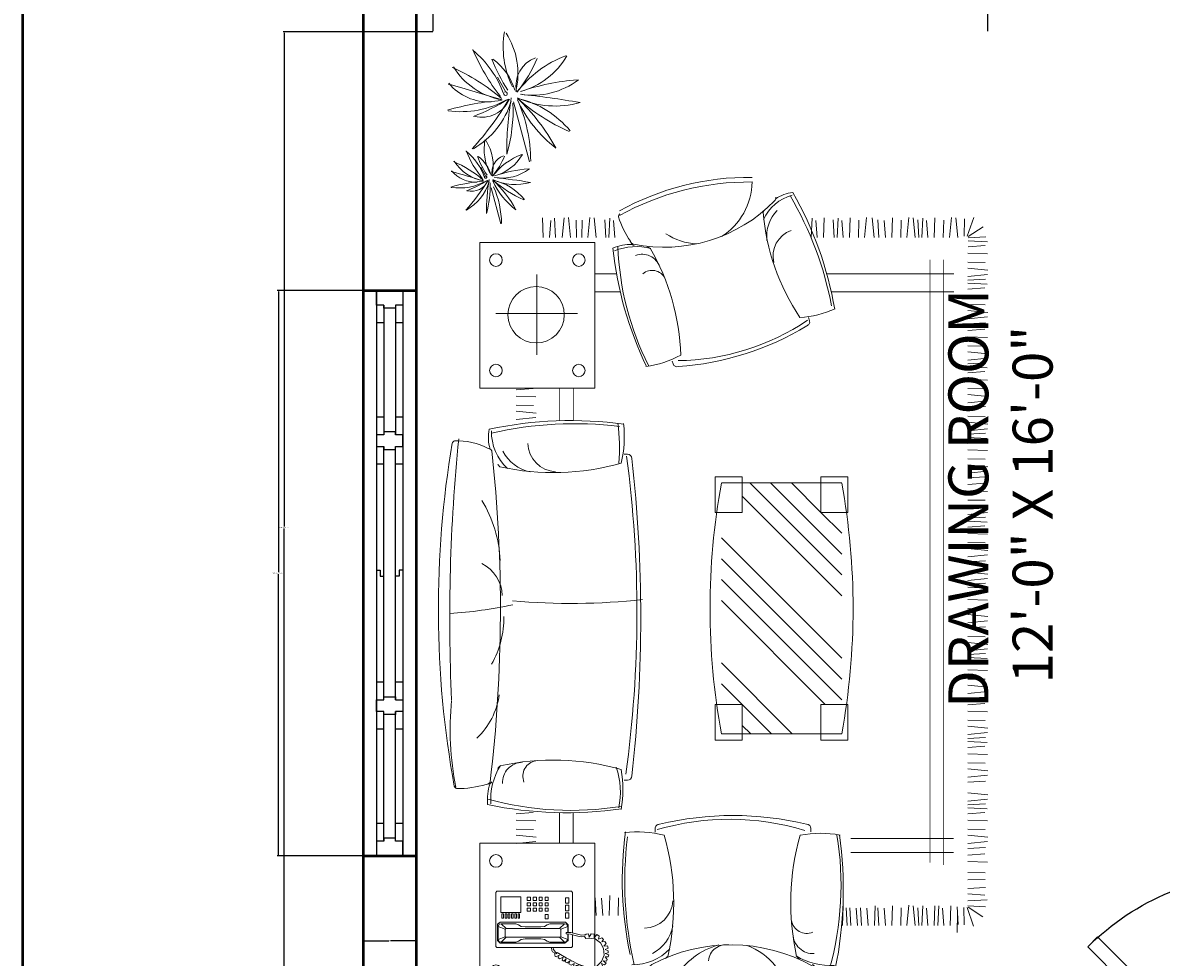
# Model space of a CAD drawing. Units: inches. Extents: x 64 to 1167, y 117 to 939.
# Tile 2 of 56: x 64 to 258, y 272 to 431. Entities that reach past the tile are written whole.
import ezdxf

# ---------------------------------------------------------------- set-up
doc = ezdxf.new("R2010")
doc.units = ezdxf.units.IN
doc.header["$MEASUREMENT"] = 0
for name, color, linetype, lineweight in [('A-ANNO-DIMS', 2, 'Continuous', 18), ('A-ANNO-TEXT', 7, 'Continuous', 25), ('A-ANNO-TTLB', 7, 'Continuous', 50), ('A-DOOR', 4, 'Continuous', 25), ('A-FURN', 8, 'Continuous', 18), ('A-GLAZ', 4, 'Continuous', 25), ('A-WALL', 7, 'Continuous', 50)]:
    doc.layers.add(name, color=color, linetype=linetype, lineweight=lineweight)
doc.styles.get("Standard").update_dxf_attribs({"font": 'arial.ttf'})
doc.dimstyles.get("Standard").update_dxf_attribs({"dimtxt": 0.18, "dimasz": 0.18, "dimexe": 0.18, "dimexo": 0.0625, "dimgap": 0.09, "dimtad": 0, "dimtih": 1, "dimtoh": 1, "dimdec": 4, "dimzin": 0, "dimdsep": 46, "dimtxsty": 'Standard', "dimcen": 0.09, "dimadec": 0, "dimazin": 0, "dimtfac": 1, "dimtdec": 4, "dimtofl": 0, "dimtmove": 0, "dimatfit": 3, "dimfxl": 1, "dimtolj": 1, "dimtzin": 0, "dimarcsym": 0})

# ---------------------------------------------------------------- blocks, each defined once
blk = doc.blocks.new('A$C68901CC0')
for p, q in [((10.95, 26.62), (12.35, 28.01)), ((12.35, 28.01), (37.4, 2.95)), ((36.01, 1.56), (10.95, 26.62)), ((0, 2.95), (0, 0)), ((1.97, 2.95), (0, 2.95)), ((1.97, 0), (1.97, 2.95)), ((37.4, 2.95), (36.01, 1.56)), ((37.4, 2.95), (37.4, 0)), ((39.37, 2.95), (37.4, 2.95)), ((39.37, 0), (39.37, 2.95)), ((0, 0), (1.97, 0)), ((37.4, 0), (39.37, 0))]:
    blk.add_line(p, q)
blk.add_arc((37.4, 2.95), 35.43, 135, 180)
blk = doc.blocks.new("W-8'")
for p, q in [((0, 9), (96, 9)), ((0, 9), (0, 0)), ((96, 9), (96, 0)), ((0, 6.75), (96, 6.75)), ((2.5, 5.5), (24.5, 5.5)), ((69.5, 5.5), (26.5, 5.5)), ((93.5, 5.5), (71.5, 5.5)), ((0, 2.25), (96, 2.25)), ((2.5, 3.5), (24.5, 3.5)), ((69.5, 3.5), (26.5, 3.5)), ((93.5, 3.5), (71.5, 3.5)), ((0, 0), (96, 0))]:
    blk.add_line(p, q)
for points in [[(0, 2.25), (0, 6.75), (2.5, 6.75), (2.5, 5.5), (3, 5.5), (3, 3.5), (2.5, 3.5), (2.5, 2.25), (0, 2.25)], [(5.5, 6.75), (5.5, 5.5)], [(21.5, 6.75), (21.5, 5.5)], [(29.5, 6.75), (29.5, 5.5)], [(47.5, 6.75), (47.5, 6.125), (48.5, 6.125), (48.5, 5.5)], [(66.5, 6.75), (66.5, 5.5)], [(74.5, 6.75), (74.5, 5.5)], [(90.5, 6.75), (90.5, 5.5)], [(96, 2.25), (96, 6.75), (93.5, 6.75), (93.5, 5.5), (93, 5.5), (93, 3.5), (93.5, 3.5), (93.5, 2.25), (96, 2.25)], [(5.5, 3.5), (5.5, 2.25)], [(21.5, 3.5), (21.5, 2.25)], [(29.5, 3.5), (29.5, 2.25)], [(47.5, 2.25), (47.5, 2.875), (48.5, 2.875), (48.5, 3.5)], [(66.5, 3.5), (66.5, 2.25)], [(74.5, 3.5), (74.5, 2.25)], [(90.5, 3.5), (90.5, 2.25)]]:
    blk.add_lwpolyline(points)
for points in [[(26.5, 6.75), (24.5, 6.75), (24.5, 5.5), (24, 5.5), (24, 3.5), (24.5, 3.5), (24.5, 2.25), (26.5, 2.25), (26.5, 3.5), (27, 3.5), (27, 5.5), (26.5, 5.5)], [(69.5, 6.75), (71.5, 6.75), (71.5, 5.5), (72, 5.5), (72, 3.5), (71.5, 3.5), (71.5, 2.25), (69.5, 2.25), (69.5, 3.5), (69, 3.5), (69, 5.5), (69.5, 5.5)]]:
    blk.add_lwpolyline(points, close=True)
blk = doc.blocks.new('A$C28C76B35')
for p, q in [((66.74, 162.49, -24.36), (86.28, 162.49, -24.36)), ((66.74, 137.72, -24.36), (66.74, 162.49, -24.36)), ((86.28, 162.49, -24.36), (86.28, 137.72, -24.36)), ((65.39, 158.69, -55.71), (65.61, 158.93, -55.71)), ((65.61, 158.17, -55.71), (65.39, 158.69, -55.71)), ((65.61, 158.93, -55.71), (66.11, 158.67, -55.71)), ((66.43, 158.63, -55.71), (65.63, 157.82, -55.71)), ((65.94, 159.21, -55.71), (66.32, 159.36, -55.71)), ((66.11, 158.67, -55.71), (65.94, 159.21, -55.71)), ((66.32, 159.36, -55.71), (66.82, 158.91, -55.71)), ((67.82, 158.89, -55.71), (66.43, 158.63, -55.71)), ((66.79, 159.49, 50.88), (67.17, 159.56, 50.88)), ((66.82, 158.91, -55.71), (66.8, 159.49, -55.71)), ((67.17, 159.56, -55.71), (67.45, 159.08, -55.71)), ((67.45, 159.08, -55.71), (67.62, 159.65, -55.71)), ((67.61, 159.66, 50.88), (68.08, 159.57, 50.88)), ((69.56, 158.28, -55.71), (67.82, 158.89, -55.71)), ((68.08, 159.56, -55.71), (68.08, 159.06, -55.71)), ((68.08, 159.06, -55.71), (68.45, 159.45, -55.71)), ((68.44, 159.45, 50.88), (68.87, 159.32, 50.88)), ((68.88, 159.32, -55.71), (68.86, 158.73, -55.71)), ((68.86, 158.73, -55.71), (69.06, 159.26, -55.71)), ((69.06, 159.26, -55.71), (69.62, 159.1, -55.71)), ((69.62, 159.1, -55.71), (69.56, 158.54, -55.71)), ((69.56, 158.54, -55.71), (70.1, 158.87, -55.71)), ((70.1, 158.87, -55.71), (70.4, 158.67, -55.71)), ((70.4, 158.67, -55.71), (70.25, 158.15, -55.71)), ((64.4, 156.67, -55.71), (64.5, 157.02, -55.71)), ((65, 156.46, -55.71), (64.4, 156.67, -55.71)), ((64.5, 157.02, -55.71), (65, 157.04, -55.71)), ((64.63, 157.46, -55.71), (64.77, 157.76, -55.71)), ((65, 157.04, -55.71), (64.63, 157.46, -55.71)), ((64.77, 157.76, -55.71), (65.33, 157.7, -55.71)), ((64.85, 158.09, -55.71), (65.11, 158.39, -55.71)), ((65.33, 157.7, -55.71), (64.85, 158.09, -55.71)), ((65.11, 158.39, -55.71), (65.61, 158.17, -55.71)), ((65.63, 157.82, -55.71), (65.16, 156.74, -55.71)), ((65.16, 156.74, -55.71), (65.26, 155.63, -55.71)), ((70.64, 157.69, -55.71), (69.56, 158.28, -55.71)), ((70.25, 158.15, -55.71), (70.75, 158.43, -55.71)), ((70.79, 157.74, -55.71), (70.64, 157.69, -55.71)), ((70.75, 158.43, -55.71), (71.14, 158.22, -55.71)), ((70.83, 157.61, -55.71), (70.79, 157.74, -55.71)), ((71.59, 157.22, -55.71), (70.83, 157.61, -55.71)), ((71.14, 158.22, -55.71), (70.98, 157.72, -55.71)), ((70.98, 157.72, -55.71), (71.4, 158.06, -55.71)), ((71.4, 158.06, -55.71), (71.81, 157.87, -55.71)), ((71.81, 157.87, -55.71), (71.59, 157.37, -55.71)), ((71.59, 157.37, -55.71), (72.01, 157.76, -55.71)), ((72.59, 156.63, -55.71), (71.59, 157.22, -55.71)), ((72.01, 157.76, -55.71), (72.31, 157.61, -55.71)), ((72.31, 157.61, -55.71), (72.14, 157.07, -55.71)), ((72.14, 157.07, -55.71), (72.68, 157.37, -55.71)), ((73.15, 156.29, -55.71), (72.59, 156.63, -55.71)), ((72.68, 157.37, -55.71), (72.96, 157.22, -55.71)), ((72.96, 157.22, -55.71), (72.81, 156.74, -55.71)), ((72.81, 156.74, -55.71), (73.3, 157.04, -55.71)), ((73.3, 157.04, -55.71), (73.5, 156.96, -55.71)), ((73.5, 156.96, -55.71), (73.56, 156.76, -55.71)), ((73.56, 156.76, -55.71), (73.57, 156.42, -55.71)), ((64.46, 156.33, -55.71), (65, 156.46, -55.71)), ((64.5, 156.02, -55.71), (64.46, 156.33, -55.71)), ((65, 155.79, -55.71), (64.5, 156.02, -55.71)), ((64.5, 155.55, -55.71), (65, 155.79, -55.71)), ((64.61, 155.16, -55.71), (64.5, 155.55, -55.71)), ((65.22, 155.22, -55.71), (64.61, 155.16, -55.71)), ((64.85, 154.77, -55.71), (65.22, 155.22, -55.71)), ((65.07, 154.42, -55.71), (64.85, 154.77, -55.71)), ((65.26, 155.63, -55.71), (65.78, 154.64, -55.71)), ((65.78, 154.64, -55.71), (66.67, 153.94, -55.71)), ((70.72, 155.44, -55.71), (70.54, 155.25, -55.71)), ((70.54, 155.25, -55.71), (70.54, 153.28, -55.71)), ((83.37, 155.44, -55.71), (70.72, 155.44, -55.71)), ((71.82, 154.7, -55.71), (71.27, 154.24, -55.71)), ((82.82, 154.7, -55.71), (71.82, 154.7, -55.71)), ((73.33, 156.52, -55.71), (73.15, 156.29, -55.71)), ((73.33, 156.33, -55.71), (73.33, 156.52, -55.71)), ((73.44, 156.22, -55.71), (73.33, 156.33, -55.71)), ((73.61, 155.98, -55.71), (73.44, 156.22, -55.71)), ((73.57, 156.42, -55.71), (73.93, 156.16, -55.71)), ((73.76, 155.78, -55.71), (73.61, 155.98, -55.71)), ((73.84, 155.44, -55.71), (73.76, 155.78, -55.71)), ((73.93, 156.16, -55.71), (74.06, 155.94, -55.71)), ((74.06, 155.94, -55.71), (74.11, 155.44, -55.71)), ((83.28, 154.24, -55.71), (82.82, 154.7, -55.71)), ((83.55, 155.25, -55.71), (83.37, 155.44, -55.71)), ((83.55, 146.08, -55.71), (83.55, 155.25, -55.71)), ((5.16, 149.65, -28.15), (5.22, 152.89, -28.15)), ((65.57, 154.5, -55.71), (65.07, 154.42, -55.71)), ((65.26, 154.07, -55.71), (65.57, 154.5, -55.71)), ((65.59, 153.79, -55.71), (65.26, 154.07, -55.71)), ((66.11, 154.05, -55.71), (65.59, 153.79, -55.71)), ((66, 153.49, -55.71), (66.11, 154.05, -55.71)), ((66.43, 153.25, -55.71), (66, 153.49, -55.71)), ((66.84, 153.77, -55.71), (66.43, 153.25, -55.71)), ((66.67, 153.94, -55.71), (67.84, 153.85, -55.71)), ((66.89, 153.18, -55.71), (66.84, 153.77, -55.71)), ((67.39, 153.14, -55.71), (66.89, 153.18, -55.71)), ((67.71, 153.66, -55.71), (67.39, 153.14, -55.71)), ((67.8, 153.12, -55.71), (67.71, 153.66, -55.71)), ((68.25, 153.16, -55.71), (67.8, 153.12, -55.71)), ((67.84, 153.85, -55.71), (68.26, 153.92, -55.71)), ((68.45, 153.36, -55.71), (68.25, 153.16, -55.71)), ((68.26, 153.92, -55.71), (68.51, 153.59, -55.71)), ((68.56, 153.31, -55.71), (68.45, 153.36, -55.71)), ((68.51, 153.59, -55.71), (68.99, 153.6, -55.71)), ((69.04, 153.33, -55.71), (68.56, 153.31, -55.71)), ((68.99, 153.6, -55.71), (69.43, 153.55, -55.71)), ((69.92, 153.1, -55.71), (69.04, 153.33, -55.71)), ((69.43, 153.55, -55.71), (70.31, 153.33, -55.71)), ((70.85, 152.88, -55.71), (69.92, 153.1, -55.71)), ((70.31, 153.33, -55.71), (70.9, 153.2, -55.71)), ((70.54, 152.96, -55.71), (70.54, 146.08, -55.71)), ((71.64, 152.87, -55.71), (70.85, 152.88, -55.71)), ((70.9, 153.2, -55.71), (71.64, 153.14, -55.71)), ((71.27, 154.24, -55.71), (71.27, 153.17, -55.71)), ((71.27, 152.87, -55.71), (71.27, 151.58, -55.71)), ((71.36, 154.06, -55.71), (71.54, 154.43, -55.71)), ((71.36, 153.16, -55.71), (71.36, 154.06, -55.71)), ((72.55, 153.6, -55.71), (71.36, 154.06, -55.71)), ((71.36, 151.86, -55.71), (71.36, 152.87, -55.71)), ((71.54, 154.43, -55.71), (71.91, 154.52, -55.71)), ((71.64, 153.14, -55.71), (71.64, 152.87, -55.71)), ((71.91, 154.52, -55.71), (74.39, 154.52, -55.71)), ((71.91, 154.52, -55.71), (72.74, 153.69, -55.71)), ((72.74, 153.69, -55.71), (72.55, 153.6, -55.71)), ((72.55, 153.6, -55.71), (72.55, 152.32, -55.71)), ((77.69, 153.69, -55.71), (72.74, 153.69, -55.71)), ((74.39, 154.52, -55.71), (74.84, 154.34, -55.71)), ((74.84, 154.34, -55.71), (75.3, 154.06, -55.71)), ((75.3, 154.06, -55.71), (75.94, 153.97, -55.71)), ((75.94, 153.97, -55.71), (77.69, 153.97, -55.71)), ((78.6, 153.97, -55.71), (77.69, 153.97, -55.71)), ((77.69, 153.69, -55.71), (81.81, 153.69, -55.71)), ((79.24, 154.06, -55.71), (78.6, 153.97, -55.71)), ((79.7, 154.34, -55.71), (79.24, 154.06, -55.71)), ((80.16, 154.52, -55.71), (79.7, 154.34, -55.71)), ((82.64, 154.52, -55.71), (80.16, 154.52, -55.71)), ((82.64, 154.52, -55.71), (81.81, 153.69, -55.71)), ((81.81, 153.69, -55.71), (82, 153.6, -55.71)), ((82, 153.6, -55.71), (83.19, 154.06, -55.71)), ((82, 153.6, -55.71), (82, 152.32, -55.71)), ((83, 154.43, -55.71), (82.64, 154.52, -55.71)), ((83.19, 154.06, -55.71), (83, 154.43, -55.71)), ((83.19, 151.86, -55.71), (83.19, 154.06, -55.71)), ((83.28, 151.49, -55.71), (83.28, 154.24, -55.71)), ((3.54, 148.64, -28.15), (2.43, 151.81, -28.15)), ((4.08, 148.65, -28.15), (4.03, 151.6, -28.15)), ((5.25, 148.56, -28.15), (5.08, 151.56, -28.15)), ((6.41, 151.68, -28.15), (6.3, 148.34, -28.15)), ((7.49, 151.68, -28.15), (7.72, 148.79, -28.15)), ((8.51, 151.68, -28.15), (8.34, 148.39, -28.15)), ((9.11, 151.68, -28.15), (9, 148.34, -28.15)), ((10.19, 151.68, -28.15), (10.42, 148.79, -28.15)), ((11.21, 151.68, -28.15), (11.04, 148.39, -28.15)), ((11.72, 151.68, -28.15), (11.89, 148.68, -28.15)), ((12.34, 151.68, -28.15), (12.68, 148.34, -28.15)), ((13.76, 151.68, -28.15), (13.42, 148.28, -28.15)), ((14.78, 151.68, -28.15), (14.72, 148.73, -28.15)), ((16.31, 151.68, -28.15), (16.2, 148.34, -28.15)), ((17.39, 151.68, -28.15), (17.62, 148.79, -28.15)), ((18.52, 151.68, -28.15), (18.69, 148.68, -28.15)), ((19.28, 151.68, -28.15), (19.17, 148.34, -28.15)), ((20.36, 151.68, -28.15), (20.59, 148.79, -28.15)), ((21.49, 151.68, -28.15), (21.66, 148.68, -28.15)), ((22.16, 151.68, -28.15), (22.38, 148.79, -28.15)), ((23.29, 151.68, -28.15), (23.46, 148.68, -28.15)), ((23.92, 151.68, -28.15), (24.09, 148.68, -28.15)), ((24.68, 151.68, -28.15), (24.56, 148.34, -28.15)), ((71.27, 151.58, -55.71), (71.73, 151.13, -55.71)), ((72.55, 152.32, -55.71), (71.36, 151.86, -55.71)), ((71.36, 151.86, -55.71), (71.54, 151.49, -55.71)), ((71.54, 151.49, -55.71), (71.91, 151.4, -55.71)), ((71.73, 151.13, -55.71), (82.82, 151.13, -55.71)), ((71.91, 151.4, -55.71), (72.74, 152.23, -55.71)), ((71.91, 151.4, -55.71), (74.39, 151.4, -55.71)), ((72.74, 152.23, -55.71), (72.55, 152.32, -55.71)), ((77.69, 152.23, -55.71), (72.74, 152.23, -55.71)), ((74.39, 151.4, -55.71), (74.84, 151.58, -55.71)), ((74.84, 151.58, -55.71), (75.3, 151.86, -55.71)), ((75.3, 151.86, -55.71), (75.94, 151.95, -55.71)), ((75.94, 151.95, -55.71), (77.69, 151.95, -55.71)), ((77.69, 152.23, -55.71), (81.81, 152.23, -55.71)), ((78.6, 151.95, -55.71), (77.69, 151.95, -55.71)), ((79.24, 151.86, -55.71), (78.6, 151.95, -55.71)), ((79.7, 151.58, -55.71), (79.24, 151.86, -55.71)), ((80.16, 151.4, -55.71), (79.7, 151.58, -55.71)), ((82.64, 151.4, -55.71), (80.16, 151.4, -55.71)), ((81.81, 152.23, -55.71), (82, 152.32, -55.71)), ((82.64, 151.4, -55.71), (81.81, 152.23, -55.71)), ((82, 152.32, -55.71), (83.19, 151.86, -55.71)), ((83, 151.49, -55.71), (82.64, 151.4, -55.71)), ((82.82, 151.13, -55.71), (83.28, 151.49, -55.71)), ((83.19, 151.86, -55.71), (83, 151.49, -55.71)), ((3.38, 148.57, -28.15), (0.87, 150.22, -28.15)), ((62.8, 149.98, -28.15), (62.74, 147.03, -28.15)), ((64.33, 149.98, -28.15), (64.22, 146.64, -28.15)), ((65.41, 149.98, -28.15), (65.64, 147.09, -28.15)), ((66.54, 149.98, -28.15), (66.71, 146.98, -28.15)), ((71.18, 150.48, -55.71), (71.73, 150.48, -55.71)), ((71.18, 149.57, -55.71), (71.18, 150.48, -55.71)), ((71.73, 149.57, -55.71), (71.18, 149.57, -55.71)), ((71.18, 149.2, -55.71), (71.73, 149.2, -55.71)), ((71.18, 148.28, -55.71), (71.18, 149.2, -55.71)), ((71.73, 150.48, -55.71), (71.73, 149.57, -55.71)), ((71.73, 149.2, -55.71), (71.73, 148.28, -55.71)), ((75.21, 150.58, -55.71), (74.66, 150.58, -55.71)), ((74.66, 150.58, -55.71), (74.66, 149.84, -55.71)), ((74.66, 149.84, -55.71), (75.21, 149.84, -55.71)), ((75.21, 149.29, -55.71), (74.66, 149.29, -55.71)), ((74.66, 149.29, -55.71), (74.66, 148.74, -55.71)), ((75.21, 149.84, -55.71), (75.21, 150.58, -55.71)), ((75.21, 148.74, -55.71), (75.21, 149.29, -55.71)), ((76.22, 149.29, -55.71), (75.67, 149.29, -55.71)), ((75.67, 149.29, -55.71), (75.67, 148.74, -55.71)), ((76.22, 148.74, -55.71), (76.22, 149.29, -55.71)), ((77.23, 149.29, -55.71), (76.68, 149.29, -55.71)), ((76.68, 149.29, -55.71), (76.68, 148.74, -55.71)), ((77.23, 148.74, -55.71), (77.23, 149.29, -55.71)), ((78.24, 149.29, -55.71), (77.69, 149.29, -55.71)), ((77.69, 149.29, -55.71), (77.69, 148.74, -55.71)), ((78.24, 148.74, -55.71), (78.24, 149.29, -55.71)), ((82.73, 149.48, -55.71), (79.34, 149.48, -55.71)), ((79.34, 149.48, -55.71), (79.34, 146.82, -55.71)), ((79.52, 150.48, -55.71), (79.79, 150.48, -55.71)), ((79.52, 149.75, -55.71), (79.52, 150.48, -55.71)), ((79.79, 149.75, -55.71), (79.52, 149.75, -55.71)), ((79.79, 150.48, -55.71), (79.79, 149.75, -55.71)), ((80.07, 150.48, -55.71), (80.35, 150.48, -55.71)), ((80.07, 149.75, -55.71), (80.07, 150.48, -55.71)), ((80.35, 149.75, -55.71), (80.07, 149.75, -55.71)), ((80.35, 150.48, -55.71), (80.35, 149.75, -55.71)), ((80.62, 150.48, -55.71), (80.9, 150.48, -55.71)), ((80.62, 149.75, -55.71), (80.62, 150.48, -55.71)), ((80.9, 149.75, -55.71), (80.62, 149.75, -55.71)), ((80.9, 150.48, -55.71), (80.9, 149.75, -55.71)), ((81.17, 150.48, -55.71), (81.45, 150.48, -55.71)), ((81.17, 149.75, -55.71), (81.17, 150.48, -55.71)), ((81.45, 149.75, -55.71), (81.17, 149.75, -55.71)), ((81.45, 150.48, -55.71), (81.45, 149.75, -55.71)), ((81.72, 150.48, -55.71), (82, 150.48, -55.71)), ((81.72, 149.75, -55.71), (81.72, 150.48, -55.71)), ((82, 149.75, -55.71), (81.72, 149.75, -55.71)), ((82, 150.48, -55.71), (82, 149.75, -55.71)), ((82.27, 150.48, -55.71), (82.55, 150.48, -55.71)), ((82.27, 149.75, -55.71), (82.27, 150.48, -55.71)), ((82.55, 149.75, -55.71), (82.27, 149.75, -55.71)), ((82.55, 150.48, -55.71), (82.55, 149.75, -55.71)), ((82.73, 146.82, -55.71), (82.73, 149.48, -55.71)), ((3.4, 147.54, -28.15), (0.11, 147.37, -28.15)), ((3.4, 148.35, -28.15), (0.4, 148.52, -28.15)), ((71.73, 148.28, -55.71), (71.18, 148.28, -55.71)), ((71.18, 147.92, -55.71), (71.73, 147.92, -55.71)), ((71.18, 147, -55.71), (71.18, 147.92, -55.71)), ((71.73, 147, -55.71), (71.18, 147, -55.71)), ((71.73, 147.92, -55.71), (71.73, 147, -55.71)), ((74.66, 148.74, -55.71), (75.21, 148.74, -55.71)), ((74.66, 148.38, -55.71), (74.66, 147.83, -55.71)), ((75.21, 148.38, -55.71), (74.66, 148.38, -55.71)), ((74.66, 147.83, -55.71), (75.21, 147.83, -55.71)), ((75.21, 147.46, -55.71), (74.66, 147.46, -55.71)), ((74.66, 147.46, -55.71), (74.66, 146.91, -55.71)), ((74.66, 146.91, -55.71), (75.21, 146.91, -55.71)), ((75.21, 147.83, -55.71), (75.21, 148.38, -55.71)), ((75.21, 146.91, -55.71), (75.21, 147.46, -55.71)), ((75.67, 148.74, -55.71), (76.22, 148.74, -55.71)), ((75.67, 148.38, -55.71), (75.67, 147.83, -55.71)), ((76.22, 148.38, -55.71), (75.67, 148.38, -55.71)), ((75.67, 147.83, -55.71), (76.22, 147.83, -55.71)), ((76.22, 147.46, -55.71), (75.67, 147.46, -55.71)), ((75.67, 147.46, -55.71), (75.67, 146.91, -55.71)), ((75.67, 146.91, -55.71), (76.22, 146.91, -55.71)), ((76.22, 147.83, -55.71), (76.22, 148.38, -55.71)), ((76.22, 146.91, -55.71), (76.22, 147.46, -55.71)), ((76.68, 148.74, -55.71), (77.23, 148.74, -55.71)), ((77.23, 148.38, -55.71), (76.68, 148.38, -55.71)), ((76.68, 148.38, -55.71), (76.68, 147.83, -55.71)), ((76.68, 147.83, -55.71), (77.23, 147.83, -55.71)), ((77.23, 147.46, -55.71), (76.68, 147.46, -55.71)), ((76.68, 147.46, -55.71), (76.68, 146.91, -55.71)), ((76.68, 146.91, -55.71), (77.23, 146.91, -55.71)), ((77.23, 147.83, -55.71), (77.23, 148.38, -55.71)), ((77.23, 146.91, -55.71), (77.23, 147.46, -55.71)), ((77.69, 148.74, -55.71), (78.24, 148.74, -55.71)), ((77.69, 148.38, -55.71), (77.69, 147.83, -55.71)), ((78.24, 148.38, -55.71), (77.69, 148.38, -55.71)), ((77.69, 147.83, -55.71), (78.24, 147.83, -55.71)), ((78.24, 147.46, -55.71), (77.69, 147.46, -55.71)), ((77.69, 147.46, -55.71), (77.69, 146.91, -55.71)), ((77.69, 146.91, -55.71), (78.24, 146.91, -55.71)), ((78.24, 147.83, -55.71), (78.24, 148.38, -55.71)), ((78.24, 146.91, -55.71), (78.24, 147.46, -55.71)), ((3.4, 145.42, -28.15), (0.4, 145.25, -28.15)), ((3.4, 146.34, -28.15), (0.51, 146.57, -28.15)), ((70.54, 146.08, -55.71), (70.72, 145.9, -55.71)), ((70.72, 145.9, -55.71), (83.37, 145.9, -55.71)), ((79.34, 146.82, -55.71), (82.73, 146.82, -55.71)), ((83.37, 145.9, -55.71), (83.55, 146.08, -55.71)), ((3.4, 143.96, -28.15), (0.45, 143.9, -28.15)), ((3.4, 142.72, -28.15), (0.45, 142.77, -28.15)), ((3.4, 140.83, -28.15), (0.06, 140.94, -28.15)), ((3.4, 139.75, -28.15), (0.51, 139.52, -28.15)), ((5.88, 139.32), (23.27, 139.32)), ((3.4, 137.79, -28.15), (0.06, 137.45, -28.15)), ((3.4, 138.62, -28.15), (0.4, 138.45, -28.15)), ((86.28, 137.72, -24.36), (66.74, 137.72, -24.36)), ((70.42, 132.55, -28.15), (70.42, 137.72, -28.15)), ((72.74, 132.55, -28.15), (72.74, 137.72, -28.15)), ((80.1, 137.79, -28.15), (76.75, 137.45, -28.15)), ((3.4, 136.37, -28.15), (0, 136.71, -28.15)), ((3.4, 135.35, -28.15), (0.45, 135.41, -28.15)), ((5.88, 136.94), (23.27, 136.94)), ((30.05, 135.82, -100.22), (30.05, 135.26, -100.22)), ((56.51, 135.86, -100.22), (56.51, 135.26, -100.22)), ((80.1, 136.37, -28.15), (76.7, 136.71, -28.15)), ((80.1, 135.35, -28.15), (77.15, 135.41, -28.15)), ((3.4, 133.82, -28.15), (0.06, 133.93, -28.15)), ((80.1, 133.82, -28.15), (76.75, 133.93, -28.15)), ((3.4, 131.72, -28.15), (0.11, 131.89, -28.15)), ((3.4, 132.74, -28.15), (0.51, 132.51, -28.15)), ((80.1, 132.74, -28.15), (77.21, 132.51, -28.15)), ((3.4, 130.59, -28.15), (0.06, 130.25, -28.15)), ((3.4, 131.21, -28.15), (0.4, 131.04, -28.15)), ((3.4, 129.17, -28.15), (0, 129.51, -28.15)), ((3.4, 126.51, -28.15), (0.06, 126.17, -28.15)), ((3.4, 127.35, -28.15), (0.4, 127.18, -28.15)), ((61.75, 127.06, -100.22), (61.19, 127.06, -100.22)), ((3.4, 125.1, -28.15), (0, 125.44, -28.15)), ((3.4, 124.07, -28.15), (0.45, 124.13, -28.15)), ((3.4, 122.54, -28.15), (0.06, 122.66, -28.15)), ((3.4, 120.45, -28.15), (0.11, 120.62, -28.15)), ((3.4, 119.94, -28.15), (0.4, 119.77, -28.15)), ((3.4, 121.47, -28.15), (0.51, 121.24, -28.15)), ((3.4, 117.89, -28.15), (0, 118.23, -28.15)), ((3.4, 119.31, -28.15), (0.06, 118.97, -28.15)), ((45.26, 119.18), (24.83, 119.18)), ((33.22, 119.18), (45.26, 107.14)), ((36.76, 119.18), (41.72, 114.21)), ((40.29, 119.18), (41.72, 117.75)), ((3.4, 116.87, -28.15), (0.45, 116.93, -28.15)), ((3.4, 115.34, -28.15), (0.06, 115.46, -28.15)), ((3.4, 114.27, -28.15), (0.51, 114.04, -28.15)), ((27.62, 114.17), (45.26, 96.53)), ((41.76, 114.17), (45.26, 110.67)), ((3.4, 112.3, -28.15), (0.06, 111.96, -28.15)), ((3.4, 113.14, -28.15), (0.4, 112.97, -28.15)), ((24.83, 113.42), (45.26, 92.99)), ((3.4, 110.89, -28.15), (0, 111.23, -28.15)), ((3.4, 108.33, -28.15), (0.06, 108.45, -28.15)), ((3.4, 109.87, -28.15), (0.45, 109.92, -28.15)), ((24.83, 109.89), (45.26, 89.46)), ((3.4, 106.24, -28.15), (0.11, 106.41, -28.15)), ((3.4, 107.26, -28.15), (0.51, 107.03, -28.15)), ((24.83, 106.35), (45.26, 85.92)), ((3.4, 105.1, -28.15), (0.06, 104.76, -28.15)), ((3.4, 105.73, -28.15), (0.4, 105.56, -28.15)), ((3.4, 103.69, -28.15), (0, 104.03, -28.15)), ((3.4, 102.66, -28.15), (0.45, 102.72, -28.15)), ((3.4, 101.19, -28.15), (0.4, 101.02, -28.15)), ((3.4, 98.94, -28.15), (0, 99.28, -28.15)), ((3.4, 100.36, -28.15), (0.06, 100.02, -28.15)), ((3.4, 97.92, -28.15), (0.45, 97.98, -28.15)), ((3.4, 96.39, -28.15), (0.06, 96.5, -28.15)), ((3.4, 95.31, -28.15), (0.51, 95.09, -28.15)), ((24.83, 95.74), (41.72, 78.86)), ((3.4, 93.16, -28.15), (0.06, 92.82, -28.15)), ((3.4, 94.29, -28.15), (0.11, 94.46, -28.15)), ((3.4, 93.78, -28.15), (0.4, 93.61, -28.15)), ((3.4, 91.74, -28.15), (0, 92.08, -28.15)), ((24.83, 92.21), (40.44, 76.6)), ((3.4, 89.13, -28.15), (0.06, 88.79, -28.15)), ((3.4, 89.96, -28.15), (0.4, 89.79, -28.15)), ((3.4, 87.71, -28.15), (0, 88.05, -28.15)), ((24.83, 88.67), (36.9, 76.6)), ((3.4, 85.16, -28.15), (0.06, 85.27, -28.15)), ((3.4, 86.69, -28.15), (0.45, 86.75, -28.15)), ((24.83, 85.14), (28.36, 81.61)), ((3.4, 83.06, -28.15), (0.11, 83.23, -28.15)), ((3.4, 84.08, -28.15), (0.51, 83.85, -28.15)), ((3.4, 81.93, -28.15), (0.06, 81.59, -28.15)), ((3.4, 82.55, -28.15), (0.4, 82.38, -28.15)), ((28.38, 81.59), (33.37, 76.6)), ((3.4, 80.51, -28.15), (0, 80.85, -28.15)), ((3.4, 79.49, -28.15), (0.45, 79.54, -28.15)), ((3.4, 77.96, -28.15), (0.06, 78.07, -28.15)), ((3.4, 75.75, -28.15), (0.4, 75.58, -28.15)), ((3.4, 76.88, -28.15), (0.51, 76.65, -28.15)), ((45.26, 76.6), (24.83, 76.6)), ((3.4, 73.5, -28.15), (0, 73.84, -28.15)), ((3.4, 74.92, -28.15), (0.06, 74.58, -28.15)), ((3.4, 72.48, -28.15), (0.45, 72.54, -28.15)), ((61.79, 71.7, -100.22), (61.19, 71.7, -100.22)), ((3.4, 70.95, -28.15), (0.06, 71.06, -28.15)), ((3.4, 69.87, -28.15), (0.51, 69.64, -28.15)), ((3.4, 67.72, -28.15), (0.06, 67.38, -28.15)), ((3.4, 68.85, -28.15), (0.11, 69.02, -28.15)), ((3.4, 68.34, -28.15), (0.4, 68.17, -28.15)), ((3.4, 66.3, -28.15), (0, 66.64, -28.15)), ((80.1, 65.82, -28.15), (76.75, 65.48, -28.15)), ((3.4, 63.81, -28.15), (0.4, 63.64, -28.15)), ((3.4, 65.28, -28.15), (0.45, 65.34, -28.15)), ((80.1, 64.4, -28.15), (76.7, 64.74, -28.15)), ((3.4, 61.56, -28.15), (0, 61.9, -28.15)), ((3.4, 62.97, -28.15), (0.06, 62.63, -28.15)), ((80.1, 61.85, -28.15), (76.75, 61.96, -28.15)), ((80.1, 63.38, -28.15), (77.15, 63.43, -28.15)), ((3.4, 60.54, -28.15), (0.45, 60.59, -28.15)), ((80.1, 60.77, -28.15), (77.21, 60.54, -28.15)), ((3.4, 59, -28.15), (0.06, 59.12, -28.15)), ((3.4, 56.91, -28.15), (0.11, 57.08, -28.15)), ((3.4, 56.4, -28.15), (0.4, 56.23, -28.15)), ((3.4, 57.93, -28.15), (0.51, 57.7, -28.15)), ((53.61, 55.9, -94.33), (53.45, 56.4, -94.33)), ((3.4, 54.36, -28.15), (0, 54.7, -28.15)), ((3.4, 55.77, -28.15), (0.06, 55.43, -28.15)), ((76.6, 41.21, -28.15), (76.6, 54.86, -28.15)), ((3.4, 53.33, -28.15), (0.45, 53.39, -28.15)), ((3.4, 51.8, -28.15), (0.06, 51.92, -28.15)), ((3.4, 50.73, -28.15), (0.51, 50.5, -28.15)), ((3.4, 48.76, -28.15), (0.06, 48.42, -28.15)), ((3.4, 49.6, -28.15), (0.4, 49.43, -28.15)), ((30.47, 48.52, -94.33), (30.3, 49.05, -94.33)), ((3.4, 47.35, -28.15), (0, 47.69, -28.15)), ((69.72, 47.85, -28.15), (83.54, 47.85, -28.15)), ((3.4, 44.8, -28.15), (0.06, 44.91, -28.15)), ((3.4, 46.33, -28.15), (0.45, 46.38, -28.15)), ((3.4, 42.7, -28.15), (0.11, 42.87, -28.15)), ((3.4, 43.72, -28.15), (0.51, 43.49, -28.15)), ((5.81, 44.17, -28.15), (26.61, 44.17, -28.15)), ((62.43, 44.17, -28.15), (66.74, 44.17, -28.15)), ((3.4, 41.56, -28.15), (0.06, 41.22, -28.15)), ((3.4, 42.19, -28.15), (0.4, 42.02, -28.15)), ((5.81, 41.08, -28.15), (27.39, 41.08, -28.15)), ((63.06, 41.08, -28.15), (66.74, 41.08, -28.15)), ((3.4, 40.15, -28.15), (0, 40.49, -28.15)), ((3.4, 39.13, -28.15), (0.45, 39.18, -28.15)), ((3.4, 37.59, -28.15), (0.06, 37.71, -28.15)), ((3.37, 35.5, -28.15), (0.08, 35.67, -28.15)), ((3.37, 34.99, -28.15), (0.37, 34.82, -28.15)), ((3.37, 36.52, -28.15), (0.48, 36.29, -28.15)), ((5.14, 34.94, -28.15), (5.48, 31.6, -28.15)), ((6.56, 34.94, -28.15), (6.22, 31.54, -28.15)), ((7.58, 34.94, -28.15), (7.52, 32, -28.15)), ((9.11, 34.94, -28.15), (9, 31.6, -28.15)), ((10.19, 34.94, -28.15), (10.42, 32.05, -28.15)), ((11.21, 34.94, -28.15), (11.04, 31.66, -28.15)), ((11.72, 34.94, -28.15), (11.89, 31.94, -28.15)), ((12.34, 34.94, -28.15), (12.68, 31.6, -28.15)), ((13.76, 34.94, -28.15), (13.42, 31.54, -28.15)), ((14.78, 34.94, -28.15), (14.72, 32, -28.15)), ((16.31, 34.94, -28.15), (16.2, 31.6, -28.15)), ((17.39, 34.94, -28.15), (17.62, 32.05, -28.15)), ((18.52, 34.94, -28.15), (18.69, 31.94, -28.15)), ((19.35, 34.94, -28.15), (19.69, 31.6, -28.15)), ((20.97, 34.94, -28.15), (20.63, 31.54, -28.15)), ((22, 34.94, -28.15), (21.94, 32, -28.15)), ((23.53, 34.94, -28.15), (23.41, 31.6, -28.15)), ((24.6, 34.94, -28.15), (24.83, 32.05, -28.15)), ((25.62, 34.94, -28.15), (25.45, 31.66, -28.15)), ((26.13, 34.94, -28.15), (26.3, 31.94, -28.15)), ((27.91, 34.94, -28.15), (27.79, 31.6, -28.15)), ((28.98, 34.94, -28.15), (29.21, 32.05, -28.15)), ((30, 34.94, -28.15), (29.83, 31.66, -28.15)), ((63.37, 34.94, -28.15), (63.59, 32.05, -28.15)), ((64.39, 34.94, -28.15), (64.22, 31.66, -28.15)), ((64.9, 34.94, -28.15), (65.07, 31.94, -28.15)), ((66.5, 34.94, -28.15), (66.84, 31.6, -28.15)), ((67.92, 34.94, -28.15), (67.58, 31.54, -28.15)), ((68.94, 34.94, -28.15), (68.88, 32, -28.15)), ((69.86, 34.94, -28.15), (69.92, 32, -28.15)), ((70.88, 34.94, -28.15), (71.22, 31.54, -28.15)), ((72.3, 34.94, -28.15), (71.96, 31.6, -28.15)), ((73.43, 34.94, -28.15), (73.6, 31.66, -28.15)), ((74.45, 34.94, -28.15), (74.23, 32.05, -28.15)), ((75.53, 34.94, -28.15), (75.65, 31.6, -28.15)), ((3.35, 34.77, -28.15), (0.84, 33.12, -28.15)), ((3.51, 34.7, -28.15), (2.4, 31.53, -28.15)), ((4.05, 34.69, -28.15), (3.99, 31.74, -28.15)), ((84.35, 26.53), (82.71, 32.62)), ((85.29, 24.48), (86.11, 23.01)), ((80.55, 11.91), (77.83, 22.07)), ((81.92, 10.16), (83.28, 7.71))]:
    blk.add_line(p, q)
at = {"const_width": 0.103, "elevation": -28.15}
for points in [[(7.54, 38.72), (7.54, 141.44)], [(9.86, 38.72), (9.86, 141.05)], [(70.42, 60.52), (70.42, 66.01)], [(72.74, 60.52), (72.74, 66.04)]]:
    blk.add_lwpolyline(points, dxfattribs=at)
for points in [[(23.79, 120.22), (23.79, 114.17), (28.38, 114.17), (28.38, 120.22)], [(46.31, 120.22), (46.31, 114.17), (41.72, 114.17), (41.72, 120.22)], [(23.79, 75.56), (23.79, 81.61), (28.38, 81.61), (28.38, 75.56)], [(46.31, 75.56), (46.31, 81.61), (41.72, 81.61), (41.72, 75.56)]]:
    blk.add_lwpolyline(points, close=True)
at = {"elevation": -24.36}
blk.add_lwpolyline([(86.28, 60.52), (86.28, 35.76), (66.74, 35.76), (66.74, 60.52)], close=True, dxfattribs=at)
for centre, radius in [((69.47, 159.47, -27.2), 1.07), ((83.55, 159.47, -27.2), 1.07), ((69.47, 140.74, -27.2), 1.07), ((83.55, 140.74, -27.2), 1.07), ((69.47, 57.51, -27.2), 1.07), ((83.55, 57.51, -27.2), 1.07), ((76.72, 48.04, -28.15), 4.79), ((69.47, 38.77, -27.2), 1.07), ((83.55, 38.77, -27.2), 1.07)]:
    blk.add_circle(centre, radius)
for centre, radius, start, end in [((44.19, 123.6, -100.22), 43.8, 71.1157, 110.2204), ((29.35, 164.01, -100.22), 0.74, 113.3322, 161.3637), ((29.34, 164.01, -100.22), 0.74, 114.0758, 156.3315), ((38.67, 116, -100.22), 49.39, 84.253, 101.4358), ((48.54, 128.59, -100.22), 36.87, 73.3816, 97.55), ((47.45, 164.2, -100.22), 11.31, 332.1884, 2.3768), ((58.09, 164.35, -100.22), 0.74, 25.7033, 68.2144), ((45.92, 164.21, -100.22), 17.27, 179.879, 196.6328), ((42.56, 166.77, -100.22), 12.19, 284.9836, 329.7062), ((90.3, 145.69, -100.22), 65.74, 168.3019, 188.2166), ((77.92, 144.85, -100.22), 52.97, 164.4911, 189.2138), ((26.82, 151.23, -100.22), 7.84, 69.9615, 96.5551), ((26.79, 147.45, -100.22), 11.05, 58.4292, 93.73), ((30.11, 159.24, -100.22), 0.74, 177.437, 237.6208), ((30.11, 159.24, -100.22), 0.74, 178.0201, 240.7828), ((30.13, 158.98, -100.22), 0.74, 184.7243, 243.4779), ((43.65, 183.47, -100.22), 28.49, 240.7828, 298.0488), ((44.46, 165.16, -100.22), 10.65, 217.955, 250.4125), ((56.72, 158.98, -100.22), 0.74, 296.5221, 355.2757), ((59.4, 151.99, -100.22), 6.91, 78.8784, 107.2062), ((-8.4, 147.85, -100.22), 41.89, 344.0709, 12.558), ((27.78, 151.92, -100.22), 6.89, 46.9453, 51.4779), ((44.45, 157.99, -100.22), 3.03, 261.0221, 354.0715), ((95.25, 147.85, -100.22), 41.89, 167.442, 195.9291), ((60.3, 149.77, -100.22), 8.6, 88.8733, 136.7696), ((59.08, 151.92, -100.22), 6.89, 128.5221, 133.0547), ((-1.21, 144.26, -100.22), 62.88, 353.0352, 12.9689), ((1.44, 143.99, -93.67), 60.65, 352.251, 12.0202), ((29.69, 153.06, -100.22), 3.42, 1.0101, 93.44), ((60.19, 150.44, -100.22), 6.82, 118.0169, 168.7258), ((30.77, 150.41, -100.22), 2.64, 9.3795, 112.5496), ((58.46, 147.21, -100.22), 4.97, 91.587, 176.7541), ((28.42, 155.21, -100.22), 19.15, 260.0867, 280.4034), ((43.86, 177.65, -100.22), 43.98, 253.1262, 286.2615), ((59.55, 154.82, -100.22), 19.01, 256.0947, 276.4886), ((30.79, 135.26, -100.22), 0.74, 180, 270), ((43.28, 185.98, -100.22), 52.95, 256.3605, 283.6395), ((55.77, 135.26, -100.22), 0.74, 270, 0), ((81.13, 128.7, -100.22), 19.15, 170.0867, 190.4034), ((71.62, 66.82, -100.22), 65.74, 78.3019, 98.2166), ((70.78, 79.2, -100.22), 52.97, 74.4911, 99.2138), ((75.46, 129, -100.22), 13.05, 167.8205, 198.7312), ((73.38, 130.33, -100.22), 11.05, 328.4292, 3.73), ((77.16, 130.3, -100.22), 7.84, 339.9615, 6.5551), ((78.99, 127.42, -100.22), 3.42, 271.0101, 3.44), ((84.91, 126.98, -100.22), 0.74, 94.7243, 153.4779), ((85.17, 127.01, -100.22), 0.74, 88.0201, 150.7828), ((85.17, 127.01, -100.22), 0.74, 87.437, 147.6208), ((90.14, 111.2, -100.22), 17.27, 89.879, 106.6328), ((89.94, 127.77, -100.22), 0.74, 23.3322, 71.3637), ((89.94, 127.77, -100.22), 0.74, 24.0758, 66.3315), ((41.93, 118.44, -100.22), 49.39, 354.253, 11.4358), ((-75.74, 97.97, -100.22), 169.06, 350.4205, 10.2522), ((302.75, 99.38, -100.22), 243.79, 173.655, 186.345), ((260.09, 98.53, -100.22), 200.49, 172.1196, 187.596), ((61.19, 126.32, -100.22), 0.74, 90, 180), ((76.34, 126.34, -100.22), 2.64, 279.3795, 22.5496), ((329.06, 98.05, -100.22), 246.28, 173.1624, 186.27), ((73.78, 165.51, -100.22), 41.89, 254.0709, 282.558), ((77.85, 129.34, -100.22), 6.89, 316.9453, 321.4779), ((95.22, 110.9, -100.22), 12.34, 133.01, 172.2904), ((141.08, 97.89), 118.18, 169.6234, 190.3766), ((-70.99, 97.89), 118.18, 349.6234, 10.3766), ((-209.5, 99.53, -100.22), 300.89, 354.1986, 2.6453), ((98.04, 99.49, -100.22), 15.84, 150.296, 180.7853), ((96.43, 23.12, -100.22), 75.81, 93.8125, 101.9792), ((70.78, -11.61, -100.22), 108.66, 84.7609, 96.4092), ((88.76, 95.88, -100.22), 6.3, 181.4899, 243.2939), ((103.9, 90.63, -100.22), 21.1, 182.4337, 211.6473), ((73.78, 32.95, -100.22), 41.89, 77.442, 105.9291), ((73.14, 69.74, -100.22), 4.97, 1.587, 86.7541), ((76.37, 68.01, -100.22), 6.82, 28.0169, 78.7258), ((75.7, 67.9, -100.22), 8.6, 358.8733, 46.7696), ((77.85, 69.13, -100.22), 6.89, 38.5221, 43.0547), ((61.19, 72.44, -100.22), 0.74, 180, 270), ((80.75, 68.65, -100.22), 19.01, 166.0947, 186.4886), ((91.62, 70.42, -100.22), 29.06, 174.4394, 187.8276), ((84.91, 71.48, -100.22), 0.74, 206.5221, 265.2757), ((77.92, 68.8, -100.22), 6.91, 348.8784, 17.2062), ((90.13, 80.75, -100.22), 11.31, 242.1884, 272.3768), ((90.28, 70.11, -100.22), 0.74, 295.7033, 338.2144), ((70.19, 129.42, -100.22), 62.88, 263.0352, 282.9689), ((70.81, 132.72, -100.22), 66.71, 262.251, 282.0202), ((55.96, 8.33, -94.33), 48.63, 93.9636, 121.2426), ((60.43, 39.39, -94.33), 17.59, 97.6899, 118.0066), ((52.81, 56.19, -94.33), 0.679, 17.6031, 107.6031), ((14.22, 34.71, -94.33), 48.65, 2.0942, 26.8169), ((3.62, 30.54, -94.33), 60.37, 5.9051, 25.8197), ((53.14, 15.46, -94.33), 40.38, 90.7293, 123.8646), ((90.61, 56.05, -94.33), 38.46, 181.674, 210.1612), ((33.07, 31.09, -94.33), 17.46, 93.6978, 114.0917), ((30.95, 49.26, -94.33), 0.679, 107.6031, 197.6031), ((-0.12, 27.27, -94.33), 38.46, 5.0451, 33.5322), ((86.38, 57.57, -94.33), 61.26, 189.8541, 209.6233), ((83.32, 57.2, -94.33), 57.74, 190.6383, 210.572), ((57.03, 42.94, -94.33), 2.43, 206.9826, 310.1527), ((31.91, 38.05, -94.33), 4.57, 289.1901, 14.3572), ((58.71, 40.92, -94.33), 3.14, 198.6132, 291.0431), ((59.7, 46.63, -94.33), 10.15, 256.0323, 291.3332), ((60.07, 42.44, -94.33), 6.33, 244.5484, 249.0811), ((60.72, 43.32, -94.33), 7.2, 267.5646, 294.1582), ((31.3, 34.74, -94.33), 6.27, 315.62, 6.3289), ((54.94, 10.42, -94.33), 26.17, 78.3859, 135.6519), ((49.15, 26.22, -94.33), 9.78, 55.5581, 88.0156), ((59.97, 35.61, -94.33), 0.679, 22.3274, 81.0811), ((60.07, 35.39, -94.33), 0.679, 15.6232, 78.3859), ((60.07, 35.39, -94.33), 0.679, 15.0401, 75.224), ((47.61, 26.65, -94.33), 15.86, 17.4821, 34.236), ((51.26, 25.34, -94.33), 11.2, 122.5868, 179.1326), ((31.01, 35.3, -94.33), 7.9, 286.4764, 334.3727), ((40.56, 70.86, -94.33), 45.35, 269.3654, 299.0389), ((62.06, 31.43, -94.33), 0.679, 310.9353, 358.9668), ((62.06, 31.43, -94.33), 0.679, 311.6789, 353.9346), ((98.06, 32.62), 15.46, 180.242, 204.0498), ((32.68, 33.75, -94.33), 6.33, 326.1252, 330.6578), ((40.56, 70.07, -94.33), 45.35, 269.3654, 299.0389), ((98.27, 40.23), 20.7, 208.9098, 226.6574), ((72.44, 20.06), 12.76, 24.3367, 52.802), ((99.99, 26.39), 15.48, 163.2117, 182.6473), ((49.28, 30.88), 35.89, 350.7455, 359.9594), ((92.77, 22.99), 8.43, 119.9306, 162.9527), ((111.04, 9.82), 30.33, 137.5232, 149.4062), ((32.42, 33.6, -94.33), 6.35, 276.4815, 304.8093), ((36.7, 28.23, -94.33), 0.679, 134.1252, 192.8788), ((86.35, 34.91), 10, 220.0008, 256.4192), ((70.46, 9.72), 20.6, 48.6584, 66.0848), ((87.69, 24.02), 3.07, 75.9187, 156.4457), ((80.22, 16.76), 9.19, 65.269, 105.9092), ((92.75, 111.88), 87.59, 260.1053, 264.1165), ((96.05, 7.28), 21.1, 110.7855, 121.5789), ((89.81, 17.04), 9.49, 82.0464, 119.2724), ((84.39, 18.13), 7.3, 31.6153, 80.1372), ((174.86, 318.98), 306.91, 253.1, 254.1681), ((83.74, 52.15), 26.83, 274.1768, 286.1059), ((99.06, 40.89), 20.62, 229.6107, 246.1427), ((87, 20.22), 5.31, 40.0083, 92.7048), ((82.53, 17.12), 7.73, 81.2259, 127.0636), ((76.2, 46.59), 23.37, 274.3837, 288.8918), ((85.81, 16.94), 7.81, 105.1243, 150.0802), ((75.23, 31.26), 11.14, 290.6384, 322.9635), ((95.05, 15.72), 14.05, 141.4571, 157.4335), ((81.16, 23.92), 3.07, 290.8411, 10.5336), ((91.65, 22.65), 7.64, 166.1764, 212.74), ((89.89, 25.88), 5.74, 195.5054, 234.7561), ((76.23, 19.91), 9.31, 350.5683, 26.0168), ((68.57, 13.8), 19.57, 22.1939, 32.6137), ((85.29, 24.7), 0.188, 19.6875, 308.9221), ((95.17, 28.23), 10.31, 199.6875, 230.5302), ((70.02, 12.48), 20.14, 22.5722, 38.3507), ((103.41, 22.07), 25.77, 180.242, 204.0498), ((103.55, 36.41), 34.49, 208.9098, 226.6574), ((60.5, 2.8), 21.27, 24.3367, 52.802), ((106.42, 13.34), 25.8, 163.2117, 182.6473), ((21.91, 20.83), 59.81, 350.7455, 359.9594), ((94.38, 7.68), 14.05, 119.9306, 162.9527), ((124.84, -14.28), 50.55, 137.5232, 149.4062), ((83.69, 27.54), 16.67, 220.0008, 256.4192), ((57.2, -14.44), 34.33, 48.6584, 66.0848), ((85.93, 9.4), 5.12, 75.9187, 156.4457), ((99.85, -18.51), 35.17, 110.7855, 121.5789), ((89.46, -2.24), 15.82, 82.0464, 119.2724), ((73.46, -2.7), 15.32, 65.269, 105.9092), ((94.35, 155.84), 145.98, 260.1053, 264.1165), ((79.34, 56.28), 44.72, 274.1768, 286.1059), ((84.77, 3.07), 8.86, 40.0083, 92.7048), ((77.32, -2.11), 12.89, 81.2259, 127.0636), ((66.77, 47.02), 38.96, 274.3837, 288.8918), ((82.78, -2.4), 13.01, 105.1243, 150.0802), ((65.16, 21.46), 18.56, 290.6384, 322.9635), ((98.19, -4.43), 23.42, 141.4571, 157.4335), ((75.03, 9.22), 5.12, 290.8411, 10.5336), ((92.53, 7.12), 12.73, 166.1764, 212.74), ((89.58, 12.49), 9.57, 195.5054, 234.7561), ((54.06, -7.65), 32.61, 22.1939, 32.6137), ((81.91, 10.52), 0.314, 19.6875, 308.9221), ((98.38, 16.42), 17.18, 199.6875, 230.5302), ((80.42, -0.42), 12.16, 31.6153, 80.1372), ((231.2, 501), 511.52, 253.1, 254.1681), ((104.87, 37.51), 34.37, 229.6107, 246.1427), ((56.47, -9.85), 33.56, 22.5722, 38.3507), ((66.81, 2.54), 15.51, 350.5683, 26.0168)]:
    blk.add_arc(centre, radius, start, end)
blk = doc.blocks.new('*D74')
at = {"layer": 'A-ANNO-DIMS', "color": 0, "lineweight": -2, "transparency": 16777216}
for p, q in [((122.04, 385.66), (107.53, 385.66)), ((107.71, 385.48), (107.71, 337.85)), ((107.71, 289.84), (107.71, 337.48)), ((122.04, 289.66), (107.53, 289.66))]:
    blk.add_line(p, q, dxfattribs=at)
for points in [[(107.68, 385.48), (107.74, 385.48), (107.71, 385.66)], [(107.68, 289.84), (107.74, 289.84), (107.71, 289.66)]]:
    blk.add_solid(points, dxfattribs=at)
at = {"layer": 'Defpoints', "color": 0, "lineweight": -2, "transparency": 16777216}
for p in [(122.11, 385.66), (107.71, 289.66), (122.11, 289.66)]:
    blk.add_point(p, dxfattribs=at)
at = {"layer": 'A-ANNO-DIMS', "color": 0, "transparency": 16777216, "insert": (107.71, 337.66), "char_height": 0.18, "attachment_point": 5}
blk.add_mtext("\\A1;WINDOW W-8' 96", dxfattribs=at)
blk = doc.blocks.new('*D75')
at = {"layer": 'A-ANNO-DIMS', "color": 0, "lineweight": -2, "transparency": 16777216}
for p, q in [((122.11, 289.6), (122.11, 275.08)), ((131.11, 289.6), (131.11, 275.08)), ((122.29, 275.26), (126.46, 275.26)), ((130.93, 275.26), (126.76, 275.26))]:
    blk.add_line(p, q, dxfattribs=at)
for points in [[(122.29, 275.29), (122.29, 275.23), (122.11, 275.26)], [(130.93, 275.29), (130.93, 275.23), (131.11, 275.26)]]:
    blk.add_solid(points, dxfattribs=at)
at = {"layer": 'Defpoints', "color": 0, "lineweight": -2, "transparency": 16777216}
for p in [(122.11, 289.66), (131.11, 289.66), (131.11, 275.26)]:
    blk.add_point(p, dxfattribs=at)
at = {"layer": 'A-ANNO-DIMS', "color": 0, "transparency": 16777216, "insert": (126.61, 275.26), "char_height": 0.18, "attachment_point": 5}
blk.add_mtext('\\A1;9', dxfattribs=at)
blk = doc.blocks.new('*D82')
at = {"layer": 'A-ANNO-DIMS', "color": 0, "lineweight": -2, "transparency": 16777216}
for p, q in [((133.91, 429.56), (108.54, 429.56)), ((108.72, 429.38), (108.72, 345.6)), ((108.72, 261.45), (108.72, 345.23)), ((133.91, 261.27), (108.54, 261.27))]:
    blk.add_line(p, q, dxfattribs=at)
for points in [[(108.69, 429.38), (108.75, 429.38), (108.72, 429.56)], [(108.69, 261.45), (108.75, 261.45), (108.72, 261.27)]]:
    blk.add_solid(points, dxfattribs=at)
at = {"layer": 'Defpoints', "color": 0, "lineweight": -2, "transparency": 16777216}
for p in [(133.97, 429.56), (108.72, 261.27), (133.97, 261.27)]:
    blk.add_point(p, dxfattribs=at)
at = {"layer": 'A-ANNO-DIMS', "color": 0, "transparency": 16777216, "insert": (108.72, 345.42), "char_height": 0.18, "attachment_point": 5}
blk.add_mtext('\\A1;SOFA SET 168', dxfattribs=at)
blk = doc.blocks.new('*D83')
at = {"layer": 'A-ANNO-DIMS', "color": 0, "lineweight": -2, "transparency": 16777216}
for p, q in [((133.97, 429.63), (133.97, 454.99)), ((134.15, 454.81), (180.86, 454.81)), ((228.01, 454.81), (181.3, 454.81)), ((228.19, 429.63), (228.19, 454.99))]:
    blk.add_line(p, q, dxfattribs=at)
for points in [[(134.15, 454.84), (134.15, 454.78), (133.97, 454.81)], [(228.01, 454.84), (228.01, 454.78), (228.19, 454.81)]]:
    blk.add_solid(points, dxfattribs=at)
at = {"layer": 'Defpoints', "color": 0, "lineweight": -2, "transparency": 16777216}
for p in [(133.97, 454.81), (133.97, 429.56), (228.19, 429.56)]:
    blk.add_point(p, dxfattribs=at)
at = {"layer": 'A-ANNO-DIMS', "color": 0, "transparency": 16777216, "insert": (181.08, 454.81), "char_height": 0.18, "attachment_point": 5}
blk.add_mtext('\\A1;94', dxfattribs=at)

msp = doc.modelspace()

# ---------------------------------------------------------------- linework, layer by layer
at = {"layer": 'A-ANNO-TTLB'}
msp.add_lwpolyline([(64.31, 939.22), (512.77, 939.22), (512.77, 116.55), (64.31, 116.55)], close=True, dxfattribs=at)
at = {"layer": 'A-WALL'}
for p, q in [((122.11, 863.2), (122.11, 155.2)), ((131.11, 433.2), (131.11, 241.2)), ((122.11, 385.66), (131.11, 385.66)), ((122.11, 289.66), (131.11, 289.66))]:
    msp.add_line(p, q, dxfattribs=at)

# ---------------------------------------------------------------- block references
at = {"layer": 'A-DOOR', "xscale": -1.213305874571074, "yscale": 1.213305874571074, "zscale": 1.213305874571074, "rotation": 90}
msp.add_blockref('A$C68901CC0', (279.11, 289.2), dxfattribs=at)
at = {"layer": 'A-FURN', "rotation": 180}
msp.add_blockref('A$C28C76B35', (228.19, 429.56, 28.15), dxfattribs=at)
at = {"layer": 'A-GLAZ', "rotation": 270}
msp.add_blockref("W-8'", (122.11, 385.66), dxfattribs=at)

# ---------------------------------------------------------------- texts
at = {"layer": 'A-ANNO-TEXT'}
for s, p in [('DRAWING ROOM', (228.26, 314.8)), ('  12\'-0" X 16\'-0"', (239.17, 314.8))]:
    msp.add_text(s, height=6.7927, rotation=90, dxfattribs=at).set_placement(p)

# ---------------------------------------------------------------- dimensions: what is measured, and where the dimension line sits
at = {"layer": 'A-ANNO-DIMS'}
dim = msp.add_linear_dim(base=(133.97, 454.81), p1=(228.19, 429.56), p2=(133.97, 429.56), angle=180, dimstyle='Standard', override={"dimdec": 0, "dimlfac": 1, "dimrnd": 0, "dimzin": 0, "dimdsep": 46, "dimlunit": 2}, dxfattribs=at)
dim.commit()
dim.dimension.update_dxf_attribs({"geometry": '*D83', "text_midpoint": (181.08, 454.81)})
for base, p1, p2, text, picture, middle in [((108.72, 261.27), (133.97, 429.56), (133.97, 261.27), 'SOFA SET <>', '*D82', (108.72, 345.42)), ((107.71, 289.66), (122.11, 385.66), (122.11, 289.66), "WINDOW W-8' <>", '*D74', (107.71, 337.66))]:
    dim = msp.add_linear_dim(base=base, p1=p1, p2=p2, angle=270, text=text, dimstyle='Standard', override={"dimdec": 0, "dimlfac": 1, "dimrnd": 0, "dimzin": 0, "dimdsep": 46, "dimlunit": 2}, dxfattribs=at)
    dim.commit()
    dim.dimension.update_dxf_attribs({"geometry": picture, "text_midpoint": middle})
dim = msp.add_linear_dim(base=(131.11, 275.26), p1=(122.11, 289.66), p2=(131.11, 289.66), dimstyle='Standard', override={"dimdec": 0, "dimlfac": 1, "dimrnd": 0, "dimzin": 0, "dimdsep": 46, "dimlunit": 2}, dxfattribs=at)
dim.commit()
dim.dimension.update_dxf_attribs({"geometry": '*D75', "text_midpoint": (126.61, 275.26)})

doc.saveas('drawing.dxf')
